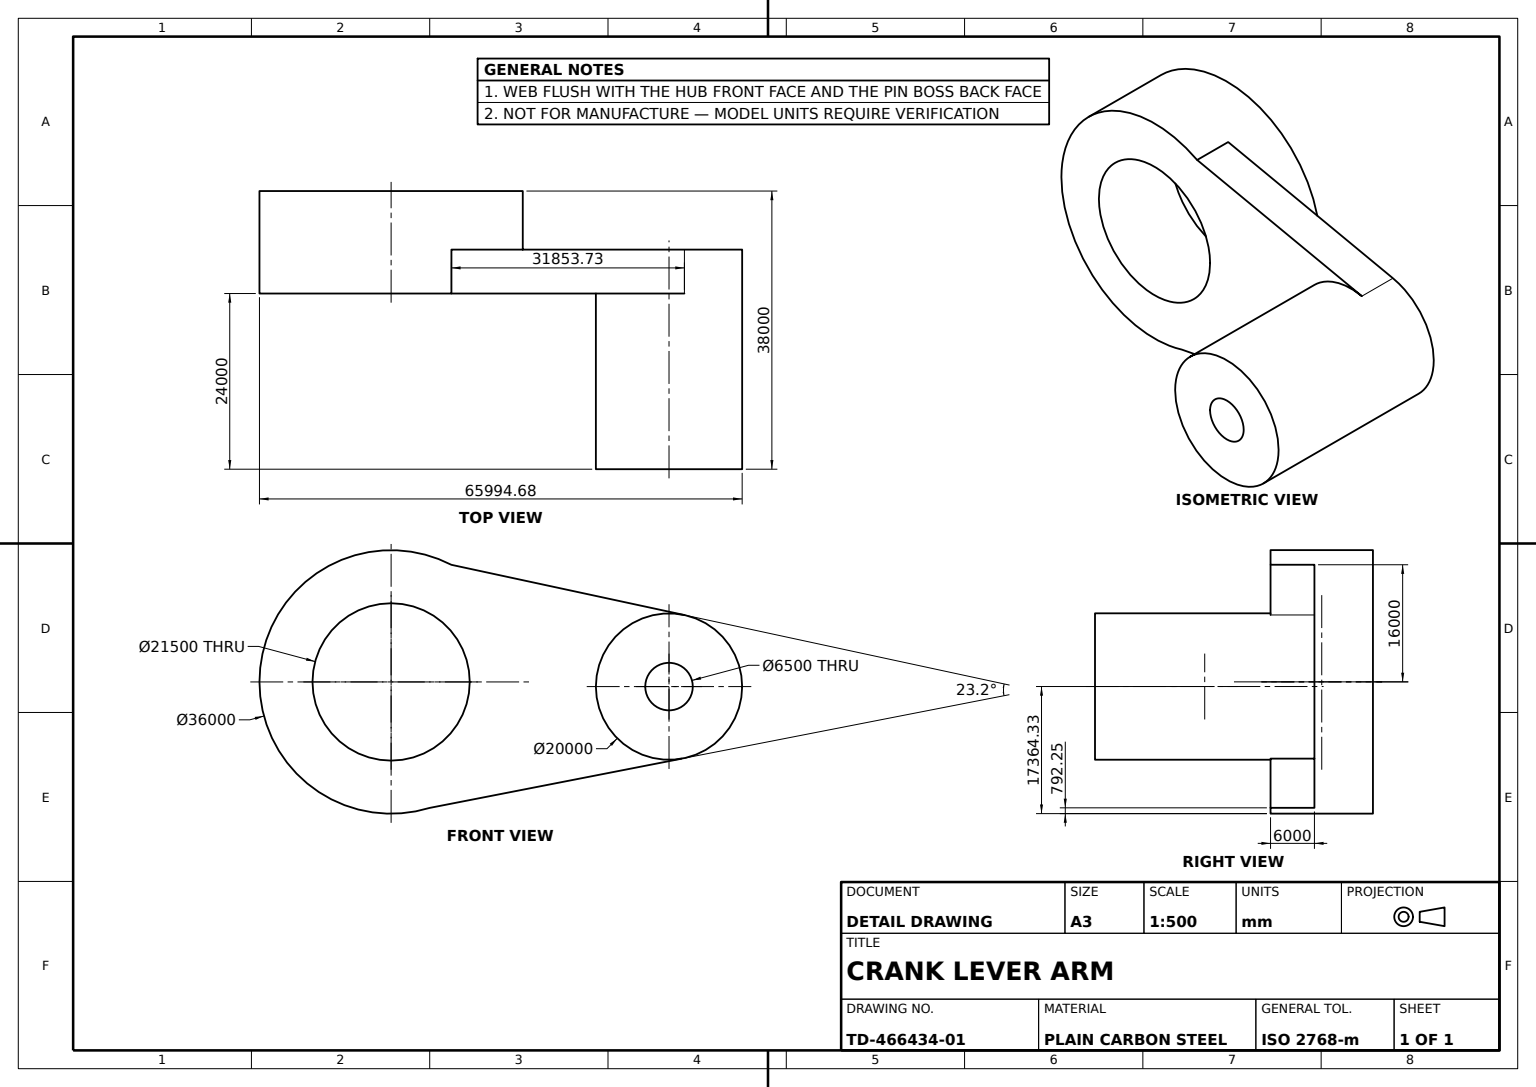
from build123d import *

# Parameters (mm, degrees)
MAIN_HUB_SKETCH_R      = 18000
MAIN_HUB_36_DEPTH      = 14000
HUB_BORE_SKETCH_R      = 10750
HUB_BORE_21_5_DEPTH    = 14000
ARM_WEB_DEPTH          = 6000
PIN_BOSS_20_DEPTH      = 24000
PIN_BOSS_20_DEPTH_BACK = 6000
PIN_BOSS_SKETCH_R      = 10000
PIN_HOLE_SKETCH_R      = 3250
PIN_HOLE_6_5_DEPTH     = 63809.225000621


with BuildPart() as part:
    # Main Hub Sketch → Main Hub Ø36 (new body)
    with BuildSketch(Plane.XY):
        Circle(MAIN_HUB_SKETCH_R)
    extrude(amount=-MAIN_HUB_36_DEPTH)

    # Hub Bore Sketch → Hub Bore Ø21.5 (cut)
    with BuildSketch(Plane(origin=(0, 0, -14000), x_dir=(-1, 0, 0), z_dir=(0, 0, -1))):
        Circle(HUB_BORE_SKETCH_R)
    extrude(amount=-HUB_BORE_21_5_DEPTH, mode=Mode.SUBTRACT)

    # Arm Web Sketch → Arm Web (add)
    with BuildSketch(Plane.XY):
        with BuildLine():
            Line((8246.211251235, 16000), (40099.945964742, 9140.210286914))
            ThreePointArc((40099.945964742, 9140.210286914), (47994.682806847, -635.671618879), (40099.945964742, -10411.553524672))
            Line((40099.945964742, -10411.553524672), (5281.400857529, -17207.754210881))
            ThreePointArc((5281.400857529, -17207.754210881), (17928.686713585, -1600.685080249), (8246.211251235, 16000))
        make_face()
    extrude(amount=-ARM_WEB_DEPTH)

    # Pin Boss Sketch → Pin Boss Ø20 (add, two sides: drawn at the far end of the back side and taken through both)
    with BuildSketch(Plane.XY.offset(-PIN_BOSS_20_DEPTH_BACK)):
        with Locations((37994.682806847, -635.671618879)):
            Circle(PIN_BOSS_SKETCH_R)
    extrude(amount=PIN_BOSS_20_DEPTH + PIN_BOSS_20_DEPTH_BACK)

    # Pin Hole Sketch → Pin Hole Ø6.5 (cut, through all)
    with BuildSketch(Plane.XY.offset(24000)):
        with Locations((37994.682806847, -635.671618879)):
            Circle(PIN_HOLE_SKETCH_R)
    extrude(amount=-PIN_HOLE_6_5_DEPTH, mode=Mode.SUBTRACT)


solid = part.part
